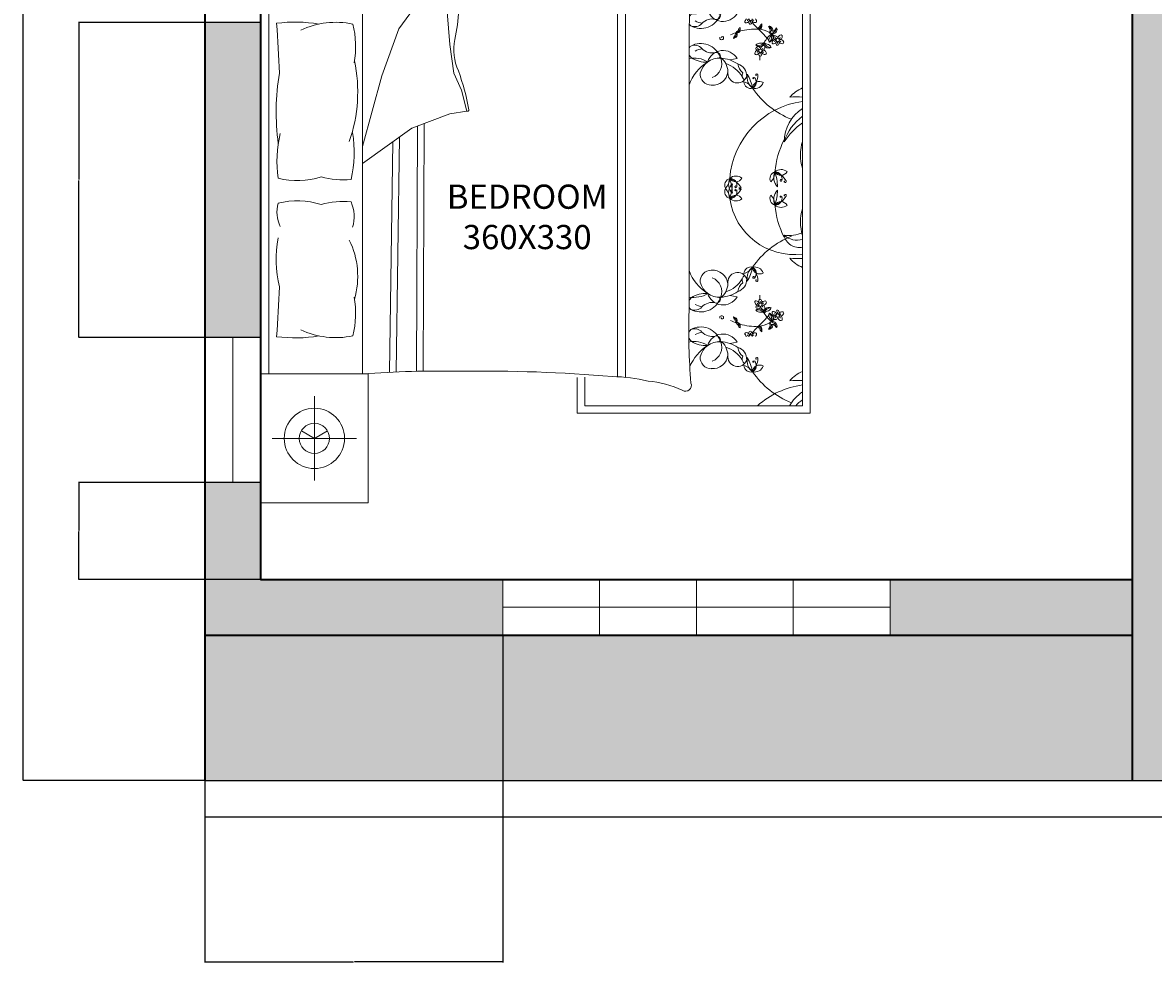
# Model space of a CAD drawing. Units: centimetres. Extents: x 2178 to 3635, y 1064 to 2635.
# Tile 1 of 9: x 2178 to 2645, y 1113 to 1502. Entities that reach past the tile are written whole.
import ezdxf

# ---------------------------------------------------------------- set-up
doc = ezdxf.new("R2010")
doc.units = ezdxf.units.CM
for name, color, linetype, lineweight in [('A-ANNO-DIMS', 2, 'Continuous', 18), ('A-AREA-IDEN', 7, 'Continuous', 18), ('A-FLOR', 7, 'Continuous', 25), ('A-FLOR-PATT', 95, 'Continuous', 13), ('A-FURN', 42, 'Continuous', 18), ('A-GLAZ', 4, 'Continuous', 18), ('A-WALL', 7, 'Continuous', 35)]:
    doc.layers.add(name, color=color, linetype=linetype, lineweight=lineweight)
doc.layers.add('A-WALL-PATT', color=18, linetype='Continuous', lineweight=13, true_color=0x000000)
doc.styles.get("Standard").update_dxf_attribs({"font": 'arial.ttf'})
doc.dimstyles.get("Standard").update_dxf_attribs({"dimtxt": 0.18, "dimasz": 0.18, "dimexe": 0.18, "dimexo": 0.0625, "dimgap": 0.09, "dimtad": 0, "dimtih": 1, "dimtoh": 1, "dimdec": 4, "dimzin": 0, "dimdsep": 46, "dimtxsty": 'Standard', "dimcen": 0.09, "dimadec": 0, "dimazin": 0, "dimtfac": 1, "dimtdec": 4, "dimtofl": 0, "dimtmove": 0, "dimatfit": 3, "dimfxl": 1, "dimtolj": 1, "dimtzin": 0, "dimarcsym": 0})

# ---------------------------------------------------------------- blocks, each defined once
blk = doc.blocks.new('bed')
for p, q in [((2798.77, 2937.13), (3098.77, 2937.13)), ((2858.77, 2937.13), (2858.77, 2854.79)), ((2828.77, 2892.53), (2828.77, 2931.73)), ((3038.77, 2933.28), (2858.77, 2933.28)), ((3068.77, 2892.53), (3068.77, 2931.73)), ((2848.37, 2912.13), (2809.17, 2912.13)), ((3049.17, 2912.13), (3088.37, 2912.13)), ((2858.77, 2889.72), (3038.77, 2889.72)), ((2900.44, 2880.8), (2933.16, 2889.72)), ((2941.19, 2889.72), (2924.75, 2866.84)), ((2878.57, 2872.91), (2900.44, 2880.8)), ((2867.02, 2864.41), (2878.57, 2872.91)), ((3037.85, 2874.18), (2928.92, 2872.64)), ((3037.97, 2877.26), (2931.16, 2875.76)), ((2924.75, 2866.84), (2918.06, 2849.23)), ((2856.09, 2851.66), (2867.02, 2864.41)), ((3037.71, 2861.65), (2922.6, 2861.18)), ((3037.69, 2864.73), (2923.78, 2864.28)), ((2858.52, 2849.23), (2856.09, 2851.66)), ((2870.67, 2850.44), (2858.52, 2849.23)), ((2885.86, 2849.23), (2870.67, 2850.44)), ((2899.23, 2847.41), (2885.86, 2849.23)), ((2907.13, 2843.76), (2899.23, 2847.41)), ((2918.06, 2849.23), (2916.85, 2841.33)), ((2916.85, 2841.33), (2907.13, 2843.76)), ((2838.37, 2790.07), (2855.34, 2790.07)), ((2838.37, 2682), (2838.37, 2790.07)), ((3040.44, 2790.07), (3057.08, 2790.07)), ((3057.08, 2790.07), (3057.08, 2682)), ((2855.33, 2786.59), (2841.85, 2786.59)), ((2841.85, 2786.59), (2841.85, 2685.48)), ((3053.6, 2786.59), (3040.38, 2786.59)), ((3053.6, 2685.48), (3053.6, 2786.59)), ((3040.42, 2767.62), (2855.31, 2767.62)), ((3040.13, 2771.36), (2855.32, 2771.36)), ((3009.67, 2738.15), (2887.87, 2738.15)), ((2871.41, 2715.89), (2870.75, 2719.28)), ((2892.38, 2715.89), (2893.04, 2719.28)), ((3003.07, 2715.89), (3002.41, 2719.28)), ((3024.04, 2715.89), (3024.7, 2719.28)), ((2841.85, 2685.48), (3053.6, 2685.48)), ((3057.08, 2682), (2838.37, 2682))]:
    blk.add_line(p, q)
for points in [[(2858.77, 2887.13), (2798.77, 2887.13), (2798.77, 2937.13)], [(3038.77, 2937.13), (3038.77, 2887.13), (3098.77, 2887.13), (3098.77, 2937.13)], [(2828.77, 2912.13), (2832.27, 2918.19)], [(3068.77, 2912.13), (3065.27, 2918.19)], [(2828.77, 2912.13), (2832.27, 2906.07)], [(3068.77, 2912.13), (3065.27, 2906.07)]]:
    blk.add_lwpolyline(points)
for points in [[(2876, 2929.65, 0.074897), (2876.37, 2910.06, -0.472817)], [(2947.37, 2908.96, 0.14099), (2947.97, 2928.95, 0.235245)], [(2960.18, 2908.96, -0.14099), (2959.58, 2928.95, -0.235245)], [(3021.54, 2929.65, -0.074897), (3021.18, 2910.06, 0.472817)], [(2855.46, 2824.19, 0.001242), (2855.31, 2767.26, -0.127202), (2849.3, 2738.9)], [(3040.05, 2773.72, 0.056112), (3042.23, 2757.21, 0.095341), (3046.45, 2741.32)]]:
    blk.add_lwpolyline(points, format="xyb")
for centre, radius in [((2828.77, 2912.13), 14), ((3068.77, 2912.13), 14), ((2828.77, 2912.13), 7), ((3068.77, 2912.13), 7), ((2888.74, 2705.02), 0.764), ((3006.71, 2705.02), 0.764), ((2883.74, 2696.97), 0.764), ((3011.71, 2696.97), 0.764)]:
    blk.add_circle(centre, radius)
for centre, radius, start, end in [((2917.11, 2821.09), 108.8, 82.2196, 99.497), ((2985.93, 2877.16), 52.74, 76.3427, 101.1841), ((3041.36, 5784.66), 2859.79, 266.68521, 267.14978), ((2940.09, 2876.08), 53.46, 81.5249, 103.96), ((2963.69, 2914.69), 14.84, 63.3437, 106.1026), ((2856.18, 5784.66), 2859.79, 272.85022, 273.31479), ((2914.22, 2902.19), 38.67, 155.1316, 191.7583), ((2983.32, 2902.19), 38.67, 348.2417, 24.8684), ((2912, 2898.93), 36.76, 354.0129, 15.8293), ((2995.54, 2898.93), 36.76, 164.1707, 185.9871), ((2886.7, 2933.16), 40.2, 255.1039, 281.0369), ((2907.87, 2961.74), 69.73, 258.0397, 289.2615), ((2936.1, 2946.52), 52.9, 259.8617, 283.6238), ((2965.7, 2909.52), 15.9, 245.0183, 288.5407), ((2993.49, 2930.2), 38.19, 243.8761, 286.1746), ((3010.84, 2933.16), 40.2, 258.9631, 284.8961), ((3576.57, 2853.06), 539.05, 176.1, 180.9282), ((2581.02, 2844.2), 275.17, 355.8294, 1.553), ((2861.22, 2957.89), 113.22, 267.4519, 281.3392), ((2888.28, 2822.94), 24.42, 66.2616, 101.3392), ((2937.68, 2954.7), 116.34, 250.1194, 259.3383), ((2916.17, 2841.09), 0.724, 268.8623, 19.7536), ((3740.68, 2833.46), 703.17, 179.11454, 184.87351), ((3044.17, 2739.79), 2.73, 246.5219, 33.8264), ((2852.06, 2739.09), 2.77, 183.98, 297.3412), ((2884.29, 2425.86), 312.3, 89.3433, 95.6887), ((2850.89, 2717.02), 22.71, 33.6671, 63.2997), ((2881.32, 2730.53), 11.57, 145.785, 184.7304), ((2859.22, 2735.93), 12.43, 328.8218, 9.1554), ((2874.61, 2734.83), 3.61, 120.0293, 142.325), ((2868.85, 2732.7), 9.56, 289.2822, 29.1751), ((2873.09, 2735.54), 4.49, 311.5653, 23.8354), ((2874.61, 2734.83), 3.61, 44.4517, 63.558), ((2894.94, 2732.7), 9.56, 150.8249, 250.7178), ((2890.7, 2735.54), 4.49, 156.1646, 228.4347), ((2889.17, 2734.83), 3.61, 113.229, 135.5483), ((2889.17, 2734.83), 3.61, 37.675, 66.7144), ((2882.46, 2730.53), 11.57, 355.2696, 34.215), ((2904.56, 2735.93), 12.43, 169.7133, 211.1782), ((2912.89, 2717.02), 22.71, 111.4941, 146.3329), ((2982.56, 2717.02), 22.71, 33.6671, 68.5059), ((3012.99, 2730.53), 11.57, 145.785, 184.7304), ((2990.89, 2735.93), 12.43, 328.8218, 10.2867), ((3006.28, 2734.83), 3.61, 113.2856, 142.325), ((3000.51, 2732.7), 9.56, 289.2822, 29.1751), ((3006.28, 2734.83), 3.61, 44.4517, 66.7144), ((3004.75, 2735.54), 4.49, 311.5653, 23.8354), ((3018.86, 2446.37), 291.92, 85.2402, 91.8035), ((3026.6, 2732.7), 9.56, 150.8249, 250.7178), ((3022.36, 2735.54), 4.49, 156.1646, 228.4347), ((3020.84, 2734.83), 3.61, 106.6343, 135.5483), ((3020.84, 2734.83), 3.61, 37.675, 72.5814), ((3014.13, 2730.53), 11.57, 355.2696, 34.215), ((3036.23, 2735.93), 12.43, 169.249, 211.1782), ((3044.56, 2717.02), 22.71, 113.6453, 146.3329), ((2864.12, 2727.92), 5.07, 84.4856, 181.0538), ((2862.56, 2724.18), 9.02, 355.2933, 76.921), ((2880.15, 2727.58), 6.15, 131.5653, 195.1471), ((2867.4, 2730.97), 8.62, 7.436, 29.9149), ((2883.64, 2727.58), 6.15, 344.8529, 48.4347), ((2896.38, 2730.97), 8.62, 150.0851, 172.564), ((2901.22, 2724.18), 9.02, 103.079, 184.7067), ((2899.66, 2727.92), 5.07, 358.9462, 95.5144), ((2995.79, 2727.92), 5.07, 84.4856, 181.0538), ((2994.23, 2724.18), 9.02, 355.2933, 76.921), ((3011.81, 2727.58), 6.15, 131.5653, 195.1471), ((2999.07, 2730.97), 8.62, 7.436, 29.9149), ((3015.3, 2727.58), 6.15, 344.8529, 48.4347), ((3028.05, 2730.97), 8.62, 150.0851, 172.564), ((3032.89, 2724.18), 9.02, 103.079, 184.7067), ((3031.33, 2727.92), 5.07, 358.9462, 95.5144), ((2866.2, 2727.2), 7.17, 174.9449, 262.8857), ((2869.01, 2729.92), 6.96, 201.5819, 291.4221), ((2867.69, 2722.36), 7.46, 299.9085, 73.1337), ((2872.41, 2725.49), 1.86, 257.3041, 15.1471), ((2896.09, 2722.36), 7.46, 106.8663, 240.0915), ((2891.37, 2725.49), 1.86, 164.8529, 282.6959), ((2894.77, 2729.92), 6.96, 248.5779, 338.4181), ((2897.59, 2727.2), 7.17, 277.1143, 5.0551), ((2997.86, 2727.2), 7.17, 174.9449, 262.8857), ((3000.68, 2729.92), 6.96, 201.5819, 291.4221), ((2999.36, 2722.36), 7.46, 299.9085, 73.1337), ((3004.08, 2725.49), 1.86, 257.3041, 15.1471), ((3027.76, 2722.36), 7.46, 106.8663, 240.0915), ((3023.04, 2725.49), 1.86, 164.8529, 282.6959), ((3026.44, 2729.92), 6.96, 248.5779, 338.4181), ((3029.25, 2727.2), 7.17, 277.1143, 5.0551), ((2864.55, 2715.65), 4.5, 80.264, 250.8688), ((2855.62, 2725.56), 14.16, 301.2614, 341.7045), ((2864.95, 2728.79), 8.71, 272.3591, 324.0401), ((2855.49, 2724.42), 16.1, 326.2883, 356.5076), ((2881.32, 2730.53), 11.57, 212.7011, 216.3445), ((2882.75, 2722.67), 0.578, 102.7051, 280.4384), ((2882.69, 2723.02), 0.94, 280.4384, 100.4136), ((2882.46, 2730.53), 11.57, 323.6555, 327.2989), ((2898.83, 2728.79), 8.71, 215.9599, 267.6409), ((2908.3, 2724.42), 16.1, 183.4924, 213.7117), ((2908.16, 2725.56), 14.16, 198.2955, 238.7386), ((2899.24, 2715.65), 4.5, 289.1312, 99.736), ((2951.17, 2718.35), 3.25, 63.0274, 163.8037), ((2947.89, 2725.94), 6.69, 271.4585, 315.3727), ((2954.28, 2718.35), 3.25, 16.1963, 116.9726), ((2957.56, 2725.94), 6.69, 224.6273, 268.5415), ((2996.21, 2715.65), 4.5, 80.264, 250.8688), ((2987.29, 2725.56), 14.16, 301.2614, 341.7045), ((2996.62, 2728.79), 8.71, 272.3591, 324.0401), ((2987.15, 2724.42), 16.1, 326.2883, 356.5076), ((3012.99, 2730.53), 11.57, 212.7011, 216.3445), ((3012.76, 2723.02), 0.94, 79.5864, 259.5616), ((3012.7, 2722.67), 0.578, 259.5616, 77.2949), ((3014.13, 2730.53), 11.57, 323.6555, 327.2989), ((3030.5, 2728.79), 8.71, 215.9599, 267.6409), ((3039.96, 2724.42), 16.1, 183.4924, 213.7117), ((3039.83, 2725.56), 14.16, 198.2955, 238.7386), ((3030.9, 2715.65), 4.5, 289.1312, 99.736), ((2863.47, 2717), 5.62, 265.969, 344.3045), ((2869.52, 2709.53), 5.99, 96.1662, 141.5825), ((2879.44, 2713.73), 1.58, 101.3256, 154.4621), ((2877.17, 2719.07), 4.74, 280.2588, 300.656), ((2903.55, 2707.57), 24.85, 163.5842, 183.8277), ((2876.15, 2719.06), 4.82, 308.2101, 316.3071), ((2879.11, 2715.89), 1.44, 278.3432, 4.2869), ((2878.31, 2717.16), 2.51, 300.656, 332.6341), ((2880.2, 2715.5), 0.611, 55.7657, 157.4417), ((2903.55, 2707.57), 24.85, 153.0032, 159.8941), ((2881.15, 2716.07), 0.611, 84.3784, 186.0543), ((2880.58, 2718.52), 2.51, 269.1859, 301.164), ((2881.32, 2717.22), 1.44, 237.5332, 323.4768), ((2879.92, 2721.32), 4.82, 285.5129, 293.6099), ((2883.07, 2715.9), 1.58, 87.3579, 140.4944), ((2879.43, 2720.42), 4.74, 301.164, 321.5612), ((2875.57, 2721.25), 8.46, 324.6898, 333.4936), ((2894.26, 2709.53), 5.99, 38.4175, 83.8338), ((2900.32, 2717), 5.62, 195.6955, 274.031), ((2951.1, 2680.2), 39.18, 94.4623, 172.255), ((2951.27, 2716.33), 4.34, 137.7873, 219.1145), ((2946.34, 2716.47), 3.27, 298.5391, 58.3627), ((2951.26, 2719.13), 3.2, 177.7585, 283.852), ((2950.61, 2713.61), 6.19, 45.5411, 114.3101), ((2956.25, 2745.4), 27.41, 252.593, 267.2582), ((2957.43, 2722.47), 9.91, 198.9159, 238.011), ((2954.84, 2713.61), 6.19, 65.6899, 134.4589), ((2949.2, 2745.4), 27.41, 272.7418, 287.407), ((2951.92, 2716.43), 0.424, 283.852, 219.9245), ((2952.44, 2714.47), 0.487, 238.011, 71.5592), ((2952.52, 2714.71), 0.236, 71.5592, 188.0167), ((2953.01, 2714.47), 0.487, 108.4408, 301.989), ((2952.93, 2714.71), 0.236, 351.9833, 108.4408), ((2953.49, 2716.59), 0.255, 320.1909, 256.0209), ((2948.02, 2722.47), 9.91, 301.989, 341.0841), ((2954.19, 2719.13), 3.2, 256.148, 2.2415), ((2959.11, 2716.47), 3.27, 121.6373, 241.4609), ((2954.18, 2716.33), 4.34, 320.8855, 42.2127), ((2953.08, 2689.24), 30.32, 352.8636, 81.8197), ((2995.13, 2717), 5.62, 265.969, 344.3045), ((3001.19, 2709.53), 5.99, 96.1662, 141.5825), ((3012.38, 2715.9), 1.58, 39.5056, 92.6421), ((3016.02, 2720.42), 4.74, 218.4388, 238.836), ((3019.88, 2721.25), 8.46, 206.5064, 215.3102), ((3014.13, 2717.22), 1.44, 216.5232, 302.4668), ((3014.87, 2718.52), 2.51, 238.836, 270.8141), ((3015.53, 2721.32), 4.82, 246.3901, 254.4871), ((2991.9, 2707.57), 24.85, 20.1059, 26.9968), ((3014.3, 2716.07), 0.611, 353.9457, 95.6216), ((3016.34, 2715.89), 1.44, 175.7131, 261.6568), ((3015.25, 2715.5), 0.611, 22.5583, 124.2343), ((3017.14, 2717.16), 2.51, 207.3659, 239.344), ((2991.9, 2707.57), 24.85, 356.1723, 16.4158), ((3019.3, 2719.06), 4.82, 223.6929, 231.7899), ((3018.28, 2719.07), 4.74, 239.344, 259.7412), ((3016.01, 2713.73), 1.58, 25.5379, 78.6744), ((3031.98, 2717), 5.62, 195.6955, 274.031), ((3025.93, 2709.53), 5.99, 38.4175, 83.8338), ((2860.73, 2709.42), 3.25, 92.9516, 193.728), ((2854.09, 2714.37), 6.69, 301.3827, 345.2969), ((2862.6, 2705.03), 6.19, 75.4653, 144.2343), ((2851.64, 2735.41), 27.41, 282.5173, 297.1824), ((2863.62, 2710.77), 2.76, 63.9755, 143.2681), ((2874.99, 2710.74), 1.27, 101.5637, 142.6358), ((2873.93, 2709.56), 0.764, 273.2768, 86.7232), ((2874.82, 2710.28), 0.73, 91.1081, 181.8675), ((2875.59, 2708.82), 1.58, 80.3487, 133.6538), ((2873.96, 2711.74), 1.84, 288.7263, 352.5032), ((2875.3, 2707.17), 2.5, 83.0852, 105.7171), ((2875.21, 2711.65), 0.59, 345.2356, 144.9248), ((2875.75, 2709.72), 0.658, 317.6792, 80.3487), ((2878.27, 2722.86), 8.46, 268.3264, 277.1302), ((2900.16, 2710.77), 2.76, 36.7319, 116.0245), ((2901.18, 2705.03), 6.19, 35.7657, 104.5347), ((2912.15, 2735.41), 27.41, 242.8176, 257.4827), ((2903.05, 2709.42), 3.25, 346.272, 87.0484), ((2909.69, 2714.37), 6.69, 194.7031, 238.6173), ((2992.4, 2709.42), 3.25, 92.9516, 193.728), ((2985.76, 2714.37), 6.69, 301.3827, 345.2969), ((2994.27, 2705.03), 6.19, 75.4653, 144.2343), ((2983.3, 2735.41), 27.41, 282.5173, 297.1824), ((2995.29, 2710.77), 2.76, 63.9755, 143.2681), ((3017.18, 2722.86), 8.46, 262.8698, 271.6736), ((3019.7, 2709.72), 0.658, 99.6513, 222.3208), ((3019.86, 2708.82), 1.58, 46.3462, 99.6513), ((3020.24, 2711.65), 0.59, 35.0752, 194.7644), ((3021.49, 2711.74), 1.84, 187.4968, 251.2737), ((3020.15, 2707.17), 2.5, 74.2829, 96.9148), ((3020.63, 2710.28), 0.73, 358.1325, 88.8919), ((3020.46, 2710.74), 1.27, 37.3642, 78.4363), ((3021.52, 2709.56), 0.764, 93.2768, 266.7232), ((3031.83, 2710.77), 2.76, 36.7319, 116.0245), ((3032.85, 2705.03), 6.19, 35.7657, 104.5347), ((3043.81, 2735.41), 27.41, 242.8176, 257.4827), ((3041.36, 2714.37), 6.69, 194.7031, 238.6173), ((3034.72, 2709.42), 3.25, 346.272, 87.0484), ((2812.68, 2680.2), 39.18, 7.745, 41.8856), ((2879.7, 2676.32), 39.18, 124.3865, 158.5908), ((2861.82, 2707.73), 4.34, 167.7115, 249.0387), ((2857.48, 2705.38), 3.27, 328.4633, 88.2869), ((2864.1, 2716.11), 9.91, 228.8402, 267.9352), ((2860.42, 2710.14), 3.2, 207.6827, 313.7762), ((2862.34, 2708.13), 0.424, 313.7762, 249.7183), ((2863.71, 2706.94), 0.236, 101.4834, 217.9409), ((2863.76, 2706.7), 0.487, 267.9352, 101.4834), ((2874.97, 2708.15), 1.26, 217.7621, 259.0403), ((2876.33, 2709.83), 2.32, 203.4276, 227.6104), ((2875.31, 2710.12), 1.25, 229.7889, 317.6792), ((2873.9, 2707.47), 1.78, 355.053, 68.3618), ((2875.09, 2707.37), 0.586, 232.4737, 355.053), ((2857.98, 2686.43), 28.48, 43.1541, 52.0459), ((2877.65, 2703.63), 1.58, 101.3256, 154.4621), ((2875.39, 2708.98), 4.74, 280.2588, 300.656), ((2876.48, 2712.77), 8.46, 268.3264, 277.1302), ((2874.36, 2708.97), 4.82, 308.2101, 316.3071), ((2877.32, 2705.8), 1.44, 278.3432, 4.2869), ((2876.52, 2707.06), 2.51, 300.656, 332.6341), ((2878.41, 2705.4), 0.611, 55.7657, 157.4417), ((2891.17, 2706.94), 12.46, 184.756, 209.2041), ((2909.1, 2733.46), 40.99, 222.2412, 232.1744), ((2884.75, 2705.38), 2.12, 272.8499, 356.1226), ((2882.89, 2706.16), 3.48, 304.5369, 16.3699), ((2883.26, 2704.56), 2.05, 321.7607, 7.9252), ((2887.73, 2705.18), 2.46, 127.3105, 187.9252), ((2884.34, 2705.45), 2.53, 355.0106, 41.658), ((2892.45, 2690.4), 14.94, 113.0501, 113.8477), ((2888.54, 2702.71), 2.41, 104.7558, 148.0499), ((2887.18, 2704.44), 1.51, 247.4086, 351.4386), ((2887.9, 2706.08), 1.04, 126.1046, 271.4281), ((2887.78, 2706.37), 0.749, 353.7526, 131.7054), ((2887.61, 2704.38), 0.506, 262.906, 7.132), ((2887.08, 2705.48), 1.05, 0.0645, 61.1507), ((2887.33, 2706.37), 1.2, 311.8413, 355.7877), ((2889.78, 2703.61), 1.26, 151.2196, 259.0403), ((2889.8, 2706.2), 1.27, 101.5637, 176.365), ((2889.63, 2705.74), 0.73, 91.1081, 181.8675), ((2891.14, 2705.29), 2.32, 203.4276, 227.6104), ((2890.41, 2704.28), 1.58, 80.3487, 133.6538), ((2890.12, 2705.58), 1.25, 229.7889, 317.6792), ((2888.77, 2707.2), 1.84, 288.7263, 352.5032), ((2888.71, 2702.93), 1.78, 355.053, 68.3618), ((2890.11, 2702.63), 2.5, 83.0852, 105.7171), ((2890.02, 2707.11), 0.59, 345.2356, 144.9248), ((2890.56, 2705.18), 0.658, 317.6792, 80.3487), ((2892.45, 2690.4), 14.94, 87.1071, 94.7585), ((2900.02, 2706.7), 0.487, 78.5166, 272.0648), ((2899.68, 2716.11), 9.91, 272.0648, 311.1598), ((2900.07, 2706.94), 0.236, 322.0591, 78.5166), ((2903.37, 2710.14), 3.2, 226.2238, 332.3173), ((2901.49, 2708.3), 0.255, 290.2667, 226.2271), ((2906.3, 2705.38), 3.27, 91.7131, 211.5367), ((2901.96, 2707.73), 4.34, 290.9613, 12.2885), ((2884.08, 2676.32), 39.18, 21.4092, 55.6135), ((3011.37, 2676.32), 39.18, 124.3865, 158.5908), ((2993.49, 2707.73), 4.34, 167.7115, 249.0387), ((2992.08, 2710.14), 3.2, 207.6827, 313.7762), ((2995.76, 2716.11), 9.91, 228.8402, 267.9352), ((2989.15, 2705.38), 3.27, 328.4633, 88.2869), ((2994.01, 2708.13), 0.424, 313.7762, 249.7183), ((2995.38, 2706.94), 0.236, 101.4834, 217.9409), ((2995.43, 2706.7), 0.487, 267.9352, 101.4834), ((3003, 2690.4), 14.94, 85.2415, 92.8929), ((3004.89, 2705.18), 0.658, 99.6513, 222.3208), ((3005.33, 2705.58), 1.25, 222.3208, 310.2111), ((3005.04, 2704.28), 1.58, 46.3462, 99.6513), ((3005.43, 2707.11), 0.59, 35.0752, 194.7644), ((3006.68, 2707.2), 1.84, 187.4968, 251.2737), ((3006.74, 2702.93), 1.78, 111.6382, 184.947), ((3005.34, 2702.63), 2.5, 74.2829, 96.9148), ((3005.82, 2705.74), 0.73, 358.1325, 88.8919), ((3004.31, 2705.29), 2.32, 312.3896, 336.5724), ((3005.65, 2706.2), 1.27, 3.635, 78.4363), ((3005.67, 2703.61), 1.26, 280.9597, 28.7804), ((3008.27, 2704.44), 1.51, 188.5614, 292.5914), ((3007.67, 2706.37), 0.749, 48.2946, 186.2474), ((3008.12, 2706.37), 1.2, 184.2123, 228.1587), ((3008.37, 2705.48), 1.05, 118.8493, 179.9355), ((3007.84, 2704.38), 0.506, 172.868, 277.094), ((3007.55, 2706.08), 1.04, 268.5719, 53.8954), ((3006.91, 2702.71), 2.41, 31.9501, 75.2442), ((3011.11, 2705.45), 2.53, 138.342, 184.9894), ((3010.7, 2705.38), 2.12, 183.8774, 267.1501), ((3003, 2690.4), 14.94, 66.1523, 66.9499), ((3012.56, 2706.16), 3.48, 163.6301, 235.4631), ((3007.72, 2705.18), 2.46, 352.0748, 52.6895), ((3012.19, 2704.56), 2.05, 172.0748, 218.2393), ((2986.35, 2733.46), 40.99, 307.8256, 317.7588), ((3004.28, 2706.94), 12.46, 330.7959, 355.244), ((3037.47, 2686.43), 28.48, 127.9541, 136.8459), ((3017.04, 2705.4), 0.611, 22.5583, 124.2343), ((3018.13, 2705.8), 1.44, 175.7131, 261.6568), ((3018.93, 2707.06), 2.51, 207.3659, 239.344), ((3021.09, 2708.97), 4.82, 223.6929, 231.7899), ((3020.06, 2708.98), 4.74, 239.344, 259.7412), ((3018.97, 2712.77), 8.46, 262.8698, 271.6736), ((3017.8, 2703.63), 1.58, 25.5379, 78.6744), ((3020.14, 2710.12), 1.25, 222.3208, 310.2111), ((3021.55, 2707.47), 1.78, 111.6382, 184.947), ((3020.36, 2707.37), 0.586, 184.947, 307.5263), ((3019.12, 2709.83), 2.32, 312.3896, 336.5724), ((3020.48, 2708.15), 1.26, 280.9597, 322.2379), ((3031.69, 2706.7), 0.487, 78.5166, 272.0648), ((3031.35, 2716.11), 9.91, 272.0648, 311.1598), ((3031.74, 2706.94), 0.236, 322.0591, 78.5166), ((3035.03, 2710.14), 3.2, 226.2238, 332.3173), ((3033.16, 2708.3), 0.255, 290.2667, 226.2271), ((3037.97, 2705.38), 3.27, 91.7131, 211.5367), ((3033.63, 2707.73), 4.34, 290.9613, 12.2885), ((3015.75, 2676.32), 39.18, 21.4092, 55.6135), ((3082.77, 2680.2), 39.18, 138.1144, 172.255), ((2878.18, 2700.87), 0.853, 146.8636, 236.9021), ((2890.21, 2719.66), 22.32, 235.1882, 238.8844), ((2879.65, 2702.11), 2.31, 199.4799, 267.6828), ((2879.39, 2701.23), 1.99, 212.8155, 277.3992), ((2878.23, 2699.91), 2.31, 266.9701, 338.2913), ((2879.13, 2701.31), 0.883, 238.8844, 314.2646), ((2878.94, 2699.33), 1.99, 280.3057, 17.1958), ((2878.77, 2699.13), 0.883, 306.3746, 21.7548), ((2880.21, 2699.7), 0.666, 19.3605, 201.7548), ((2880.22, 2700.2), 0.666, 311.8703, 134.2646), ((2892.74, 2694.13), 13.31, 153.7819, 158.2913), ((2882.15, 2703.22), 3.48, 247.2305, 319.0635), ((2881, 2702.05), 2.05, 264.4544, 310.6188), ((2891.17, 2706.94), 12.46, 214.0033, 222.4917), ((2882.5, 2701.23), 2.12, 218.3208, 298.8162), ((2892.45, 2690.4), 14.94, 120.544, 139.818), ((2882.9, 2698.03), 1.04, 126.1046, 271.4281), ((2882.78, 2698.31), 0.749, 353.7526, 131.7054), ((2883.94, 2698.62), 2.46, 70.0041, 130.6188), ((2882.35, 2701.62), 2.53, 297.7043, 344.3516), ((2884.8, 2698.15), 1.27, 101.5637, 176.365), ((2883.78, 2699.15), 1.84, 288.7263, 352.5032), ((2885.03, 2699.06), 0.59, 345.2356, 144.9248), ((2883.69, 2701.61), 2.05, 8.7227, 54.8872), ((2883.8, 2699.97), 3.48, 0.278, 72.111), ((2885.36, 2701.25), 2.12, 20.5253, 88.5375), ((2888.15, 2702.29), 2.46, 188.7227, 249.3375), ((2887.13, 2703.59), 0.757, 148.0499, 225.6268), ((2884.99, 2701.06), 2.53, 334.9899, 21.6373), ((2889.9, 2702.83), 0.586, 232.4737, 355.053), ((2948.18, 2697.36), 3.25, 63.0274, 163.8037), ((2944.89, 2704.96), 6.69, 271.4585, 315.3727), ((2947.61, 2692.63), 6.19, 45.5411, 114.3101), ((2957.84, 2692.63), 6.19, 65.6899, 134.4589), ((2957.27, 2697.36), 3.25, 16.1963, 116.9726), ((2960.56, 2704.96), 6.69, 224.6273, 268.5415), ((3005.55, 2702.83), 0.586, 184.947, 307.5263), ((3010.46, 2701.06), 2.53, 158.3627, 205.0101), ((3010.09, 2701.25), 2.12, 91.4625, 159.4747), ((3011.65, 2699.97), 3.48, 107.889, 179.722), ((3007.3, 2702.29), 2.46, 290.6625, 351.2773), ((3008.32, 2703.59), 0.757, 314.3732, 31.9501), ((3011.76, 2701.61), 2.05, 125.1128, 171.2773), ((3010.42, 2699.06), 0.59, 35.0752, 194.7644), ((3011.67, 2699.15), 1.84, 187.4968, 251.2737), ((3003, 2690.4), 14.94, 40.182, 59.456), ((3011.51, 2698.62), 2.46, 49.3812, 109.9959), ((3013.3, 2703.22), 3.48, 220.9365, 292.7695), ((3013.1, 2701.62), 2.53, 195.6484, 242.2957), ((3010.65, 2698.15), 1.27, 3.635, 78.4363), ((3012.67, 2698.31), 0.749, 48.2946, 186.2474), ((3012.95, 2701.23), 2.12, 241.1838, 321.6792), ((3012.55, 2698.03), 1.04, 268.5719, 53.8954), ((3014.45, 2702.05), 2.05, 229.3812, 275.5456), ((3004.28, 2706.94), 12.46, 317.5083, 325.9967), ((3016.51, 2699.33), 1.99, 162.8042, 259.6943), ((3015.23, 2700.2), 0.666, 45.7354, 228.1297), ((3015.24, 2699.7), 0.666, 338.2452, 160.6395), ((3002.71, 2694.13), 13.31, 21.7087, 26.2181), ((3017.22, 2699.91), 2.31, 201.7087, 273.0299), ((3016.32, 2701.31), 0.883, 225.7354, 301.1156), ((3016.68, 2699.13), 0.883, 158.2452, 233.6254), ((3016.06, 2701.23), 1.99, 262.6008, 327.1845), ((3015.8, 2702.11), 2.31, 272.3172, 340.5201), ((3005.24, 2719.66), 22.32, 301.1156, 304.8118), ((3017.27, 2700.87), 0.853, 303.0979, 33.1364), ((2866.06, 2716.39), 22.32, 302.6784, 306.3746), ((2878.82, 2698.08), 0.853, 214.3538, 304.3923), ((2882.14, 2695.53), 0.757, 148.0499, 225.6268), ((2883.54, 2694.66), 2.41, 104.7558, 148.0499), ((2882.19, 2696.38), 1.51, 247.4086, 351.4386), ((2882.61, 2696.32), 0.506, 262.906, 7.132), ((2882.08, 2697.42), 1.05, 0.0645, 61.1507), ((2882.33, 2698.32), 1.2, 311.8413, 355.7877), ((2884.78, 2695.55), 1.26, 151.2196, 259.0403), ((2884.63, 2697.69), 0.73, 91.1081, 181.8675), ((2886.15, 2697.23), 2.32, 203.4276, 227.6104), ((2885.41, 2696.22), 1.58, 80.3487, 133.6538), ((2885.13, 2697.53), 1.25, 229.7889, 317.6792), ((2883.72, 2694.88), 1.78, 355.053, 68.3618), ((2885.11, 2694.58), 2.5, 83.0852, 105.7171), ((2884.9, 2694.78), 0.586, 232.4737, 355.053), ((2885.56, 2697.13), 0.658, 317.6792, 80.3487), ((2931.45, 2674.95), 19.09, 91.272, 146.5383), ((2938.32, 2671.39), 23.79, 107.8504, 143.6964), ((2950.82, 2664.7), 35.39, 124.0123, 144.053), ((2948.1, 2659.21), 39.18, 94.4623, 117.4146), ((2948.27, 2695.35), 4.34, 137.7873, 219.1145), ((2943.34, 2695.48), 3.27, 298.5391, 58.3627), ((2948.26, 2698.14), 3.2, 177.7585, 283.852), ((2954.43, 2701.48), 9.91, 198.9159, 238.011), ((2953.26, 2724.42), 27.41, 252.593, 267.2582), ((2948.92, 2695.44), 0.424, 283.852, 219.9245), ((2949.44, 2693.49), 0.487, 238.011, 71.5592), ((2949.52, 2693.73), 0.236, 71.5592, 188.0167), ((2952.19, 2724.42), 27.41, 272.7418, 287.407), ((2956.01, 2693.49), 0.487, 108.4408, 301.989), ((2955.93, 2693.73), 0.236, 351.9833, 108.4408), ((2956.49, 2695.61), 0.255, 320.1909, 256.0209), ((2951.02, 2701.48), 9.91, 301.989, 341.0841), ((2957.19, 2698.14), 3.2, 256.148, 2.2415), ((2962.11, 2695.48), 3.27, 121.6373, 241.4609), ((2957.18, 2695.35), 4.34, 320.8855, 42.2127), ((2957.35, 2659.21), 39.18, 62.5854, 85.5377), ((2957, 2692.01), 17.54, 338.117, 6.6195), ((2973.09, 2687.13), 7.03, 346.3898, 79.0739), ((2967.81, 2688.1), 8.89, 342.8609, 41.9049), ((3009.89, 2697.13), 0.658, 99.6513, 222.3208), ((3010.32, 2697.53), 1.25, 222.3208, 310.2111), ((3010.04, 2696.22), 1.58, 46.3462, 99.6513), ((3011.73, 2694.88), 1.78, 111.6382, 184.947), ((3010.55, 2694.78), 0.586, 184.947, 307.5263), ((3010.34, 2694.58), 2.5, 74.2829, 96.9148), ((3010.82, 2697.69), 0.73, 358.1325, 88.8919), ((3009.3, 2697.23), 2.32, 312.3896, 336.5724), ((3010.67, 2695.55), 1.26, 280.9597, 28.7804), ((3013.26, 2696.38), 1.51, 188.5614, 292.5914), ((3013.12, 2698.32), 1.2, 184.2123, 228.1587), ((3013.37, 2697.42), 1.05, 118.8493, 179.9355), ((3012.84, 2696.32), 0.506, 172.868, 277.094), ((3011.91, 2694.66), 2.41, 31.9501, 75.2442), ((3013.31, 2695.53), 0.757, 314.3732, 31.9501), ((3029.39, 2716.39), 22.32, 233.6254, 237.3216), ((3016.63, 2698.08), 0.853, 235.6077, 325.6462), ((2832.33, 2674.95), 19.09, 33.4617, 60.1116), ((2825.46, 2671.39), 23.79, 36.3036, 46.4814), ((2843.02, 2679.37), 15.93, 22.5547, 48.9546), ((2799.39, 2687.93), 54.2, 357.4081, 3.6519), ((2920.76, 2679.37), 15.93, 131.0454, 157.4453), ((2964.39, 2687.93), 54.2, 176.3481, 182.5919), ((2931.06, 2687.93), 54.2, 357.4081, 3.6519), ((2974.69, 2679.37), 15.93, 22.5547, 48.9546), ((3052.43, 2679.37), 15.93, 131.0454, 157.4453), ((3096.06, 2687.93), 54.2, 176.3481, 182.5919), ((3063.12, 2674.95), 19.09, 119.8884, 146.5383), ((3069.99, 2671.39), 23.79, 133.5186, 143.6964), ((2937.15, 2664.88), 21.54, 73.5431, 107.0202), ((2945.68, 2653.78), 31.85, 94.3787, 95.6357), ((2962.46, 2631.95), 56.92, 109.7217, 109.9028), ((2968.3, 2664.88), 21.54, 72.9798, 106.4569), ((2959.77, 2653.78), 31.85, 84.3643, 85.6213), ((2942.99, 2631.95), 56.92, 70.0972, 70.2783)]:
    blk.add_arc(centre, radius, start, end)
blk = doc.blocks.new('WIN-1600-4LT')
for p, q in [((0, 23), (0, 0)), ((40, 23), (40, 0)), ((80, 23), (80, 0)), ((120, 23), (120, 0)), ((160, 23), (160, 0)), ((0, 11.5), (160, 11.5))]:
    blk.add_line(p, q)
blk = doc.blocks.new('WIN-0600')
for p, q in [((0, 60), (23, 60)), ((11.5, 60), (11.5, 0)), ((0, 0), (23, 0))]:
    blk.add_line(p, q)
blk = doc.blocks.new('*D46')
at = {"layer": 'A-ANNO-DIMS', "color": 0, "lineweight": -2, "transparency": 16777216}
for p, q in [((2253.6, 1248.53), (2253.6, 1173.41)), ((3559.6, 1248.53), (3559.6, 1173.41)), ((2253.78, 1173.59), (2906.25, 1173.59)), ((3559.42, 1173.59), (2906.95, 1173.59))]:
    blk.add_line(p, q, dxfattribs=at)
at = {"layer": 'A-ANNO-DIMS', "color": 0, "transparency": 16777216}
for points in [[(2253.78, 1173.62), (2253.78, 1173.56), (2253.6, 1173.59)], [(3559.42, 1173.62), (3559.42, 1173.56), (3559.6, 1173.59)]]:
    blk.add_solid(points, dxfattribs=at)
at = {"layer": 'Defpoints', "color": 0, "transparency": 16777216}
for p in [(2253.6, 1248.59), (3559.6, 1248.59), (2253.6, 1173.59)]:
    blk.add_point(p, dxfattribs=at)
at = {"layer": 'A-ANNO-DIMS', "color": 0, "transparency": 16777216, "insert": (2906.6, 1173.59), "char_height": 0.18, "attachment_point": 5}
blk.add_mtext('\\A1;1306', dxfattribs=at)
blk = doc.blocks.new('*D47')
at = {"layer": 'A-ANNO-DIMS', "color": 0, "lineweight": -2, "transparency": 16777216}
for p, q in [((2511.88, 2559.59), (2178.42, 2559.59)), ((2178.6, 2559.41), (2178.6, 1874.27)), ((2178.6, 1188.77), (2178.6, 1873.91)), ((2253.54, 1188.59), (2178.42, 1188.59))]:
    blk.add_line(p, q, dxfattribs=at)
at = {"layer": 'A-ANNO-DIMS', "color": 0, "transparency": 16777216}
for points in [[(2178.57, 2559.41), (2178.63, 2559.41), (2178.6, 2559.59)], [(2178.57, 1188.77), (2178.63, 1188.77), (2178.6, 1188.59)]]:
    blk.add_solid(points, dxfattribs=at)
at = {"layer": 'Defpoints', "color": 0, "transparency": 16777216}
for p in [(2178.6, 2559.59), (2511.95, 2559.59), (2253.6, 1188.59)]:
    blk.add_point(p, dxfattribs=at)
at = {"layer": 'A-ANNO-DIMS', "color": 0, "transparency": 16777216, "insert": (2178.6, 1874.09), "char_height": 0.18, "attachment_point": 5}
blk.add_mtext('\\A1;1371', dxfattribs=at)
blk = doc.blocks.new('*D69')
at = {"layer": 'A-ANNO-DIMS', "color": 0, "lineweight": -2, "transparency": 16777216}
for p, q in [((2276.54, 1311.59), (2201.42, 1311.59)), ((2201.6, 1311.41), (2201.6, 1291.77)), ((2201.6, 1271.77), (2201.6, 1291.41)), ((2276.54, 1271.59), (2201.42, 1271.59))]:
    blk.add_line(p, q, dxfattribs=at)
at = {"layer": 'A-ANNO-DIMS', "color": 0, "transparency": 16777216}
for points in [[(2201.57, 1311.41), (2201.63, 1311.41), (2201.6, 1311.59)], [(2201.57, 1271.77), (2201.63, 1271.77), (2201.6, 1271.59)]]:
    blk.add_solid(points, dxfattribs=at)
at = {"layer": 'Defpoints', "color": 0, "transparency": 16777216}
for p in [(2201.6, 1311.59), (2276.6, 1311.59), (2276.6, 1271.59)]:
    blk.add_point(p, dxfattribs=at)
at = {"layer": 'A-ANNO-DIMS', "color": 0, "transparency": 16777216, "insert": (2201.6, 1291.59), "char_height": 0.18, "attachment_point": 5}
blk.add_mtext('\\A1;40', dxfattribs=at)
blk = doc.blocks.new('*D70')
at = {"layer": 'A-ANNO-DIMS', "color": 0, "lineweight": -2, "transparency": 16777216}
for p, q in [((2276.54, 1501.59), (2201.42, 1501.59)), ((2201.6, 1501.41), (2201.6, 1436.77)), ((2201.6, 1371.77), (2201.6, 1436.41)), ((2276.54, 1371.59), (2201.42, 1371.59))]:
    blk.add_line(p, q, dxfattribs=at)
at = {"layer": 'A-ANNO-DIMS', "color": 0, "transparency": 16777216}
for points in [[(2201.57, 1501.41), (2201.63, 1501.41), (2201.6, 1501.59)], [(2201.57, 1371.77), (2201.63, 1371.77), (2201.6, 1371.59)]]:
    blk.add_solid(points, dxfattribs=at)
at = {"layer": 'Defpoints', "color": 0, "transparency": 16777216}
for p in [(2201.6, 1501.59), (2276.6, 1501.59), (2276.6, 1371.59)]:
    blk.add_point(p, dxfattribs=at)
at = {"layer": 'A-ANNO-DIMS', "color": 0, "transparency": 16777216, "insert": (2201.6, 1436.59), "char_height": 0.18, "attachment_point": 5}
blk.add_mtext('\\A1;130', dxfattribs=at)
blk = doc.blocks.new('*D75')
at = {"layer": 'A-ANNO-DIMS', "color": 0, "lineweight": -2, "transparency": 16777216}
for p, q in [((2253.6, 1248.53), (2253.6, 1113.41)), ((2376.6, 1248.53), (2376.6, 1113.41)), ((2253.78, 1113.59), (2314.82, 1113.59)), ((2376.42, 1113.59), (2315.39, 1113.59))]:
    blk.add_line(p, q, dxfattribs=at)
at = {"layer": 'A-ANNO-DIMS', "color": 0, "transparency": 16777216}
for points in [[(2253.78, 1113.62), (2253.78, 1113.56), (2253.6, 1113.59)], [(2376.42, 1113.62), (2376.42, 1113.56), (2376.6, 1113.59)]]:
    blk.add_solid(points, dxfattribs=at)
at = {"layer": 'Defpoints', "color": 0, "transparency": 16777216}
for p in [(2253.6, 1248.59), (2376.6, 1248.59), (2376.6, 1113.59)]:
    blk.add_point(p, dxfattribs=at)
at = {"layer": 'A-ANNO-DIMS', "color": 0, "transparency": 16777216, "insert": (2315.1, 1113.59), "char_height": 0.18, "attachment_point": 5}
blk.add_mtext('\\A1;123', dxfattribs=at)

msp = doc.modelspace()

# ---------------------------------------------------------------- hatches: boundary and pattern name
at = {"layer": 'A-FLOR-PATT'}
h = msp.add_hatch(color=256, dxfattribs=at)
h.dxf.hatch_style = 1
h.paths.add_polyline_path([(3559.605, 1741.59), (3395.605, 1741.59), (3395.605, 1623.59), (3559.605, 1623.59)])
h.paths.add_polyline_path([(3536.605, 1248.59), (3395.605, 1248.59), (3395.605, 1188.59), (3536.605, 1188.59)])
h.paths.add_polyline_path([(2636.605, 1248.59), (2253.605, 1248.59), (2253.605, 1188.59), (2636.605, 1188.59)])
at = {"layer": 'A-WALL-PATT'}
h = msp.add_hatch(color=256, dxfattribs=at)
h.dxf.hatch_style = 1
h.paths.add_polyline_path([(2276.605, 2499.59), (2253.605, 2499.59), (2253.605, 2476.59), (2276.605, 2476.59)])
h.paths.add_polyline_path([(2411.605, 2350.59), (2253.605, 2350.59), (2253.605, 2327.59), (2411.605, 2327.59)])
h.paths.add_polyline_path([(2276.605, 2252.59), (2253.605, 2252.59), (2253.605, 2020.59), (2276.605, 2020.59), (2276.605, 2093.59), (2561.605, 2093.59), (2561.605, 2116.59), (2276.605, 2116.59)])
h.paths.add_polyline_path([(2659.605, 1787.59), (2610.616, 1787.59), (2276.605, 1787.59), (2276.605, 1860.59), (2253.605, 1860.59), (2253.605, 1732.09), (2276.605, 1732.09), (2276.605, 1764.59), (2516.605, 1764.59), (2516.605, 1699.59), (2539.605, 1699.59), (2539.605, 1764.59), (2659.605, 1764.59)])
h.paths.add_polyline_path([(2539.605, 1624.59), (2276.605, 1624.59), (2276.605, 1657.09), (2253.605, 1657.09), (2253.605, 1561.59), (2276.605, 1561.59), (2276.605, 1601.59), (2539.605, 1601.59)])
h.paths.add_polyline_path([(2276.605, 1501.59), (2253.605, 1501.59), (2253.605, 1371.59), (2276.605, 1371.59)])
h.paths.add_polyline_path([(2376.605, 1271.59), (2276.605, 1271.59), (2276.605, 1311.59), (2253.605, 1311.59), (2253.605, 1248.59), (2376.605, 1248.59)])
h.paths.add_polyline_path([(2636.605, 1271.59), (2536.605, 1271.59), (2536.605, 1248.59), (2636.605, 1248.59)])
h.paths.add_polyline_path([(2659.605, 1600.59), (2919.605, 1600.59), (2919.605, 1623.59), (2636.605, 1623.59), (2636.605, 1188.59), (2659.605, 1188.59)])
h.paths.add_polyline_path([(2939.605, 1211.59), (2759.605, 1211.59), (2759.605, 1188.59), (2939.605, 1188.59)])
h.paths.add_polyline_path([(3062.605, 1288.59), (3039.605, 1288.59), (3039.605, 1188.59), (3062.605, 1188.59)])
h.paths.add_polyline_path([(3372.605, 1248.59), (3062.605, 1248.59), (3062.605, 1218.59), (3372.605, 1218.59)])
h.paths.add_polyline_path([(3395.605, 1271.59), (3372.605, 1271.59), (3372.605, 1248.59), (3395.605, 1248.59)])
h.paths.add_polyline_path([(3559.605, 1271.59), (3536.605, 1271.59), (3536.605, 1248.59), (3559.605, 1248.59)])
h.paths.add_polyline_path([(3559.605, 1623.59), (3536.605, 1623.59), (3536.605, 1600.59), (3559.605, 1600.59)])
h.paths.add_polyline_path([(3395.605, 1623.59), (3162.605, 1623.59), (3162.605, 1600.59), (3395.605, 1600.59)])
h.paths.add_polyline_path([(3395.605, 1411.59), (3277.1, 1411.59), (3277.1, 1388.59), (3395.605, 1388.59)])
h.paths.add_polyline_path([(3157.1, 1411.59), (3062.605, 1411.59), (3062.605, 1623.59), (3039.605, 1623.59), (3039.605, 1388.59), (3157.1, 1388.59)])
h.paths.add_polyline_path([(3559.605, 1797.09), (3536.605, 1797.09), (3536.605, 1764.59), (3316.605, 1764.59), (3316.605, 1927.59), (3293.605, 1927.59), (3293.605, 1741.59), (3372.605, 1741.59), (3395.605, 1741.59), (3559.605, 1741.59)])
h.paths.add_polyline_path([(3559.605, 1990.59), (3536.605, 1990.59), (3536.605, 1974.446), (3536.605, 1927.59), (3391.605, 1927.59), (3391.605, 1904.59), (3536.605, 1904.59), (3536.605, 1872.09), (3559.605, 1872.09)])
h.paths.add_polyline_path([(3559.605, 2180.59), (3536.605, 2180.59), (3536.605, 2050.59), (3559.605, 2050.59)])
h.paths.add_polyline_path([(3559.605, 2326.59), (3446.105, 2326.59), (3446.105, 2303.59), (3536.605, 2303.59), (3536.605, 2240.59), (3559.605, 2240.59)])
h.paths.add_polyline_path([(3286.105, 2326.59), (3195.605, 2326.59), (3195.605, 2499.59), (3082.605, 2499.59), (3082.605, 2476.59), (3172.605, 2476.59), (3172.605, 2116.59), (2809.605, 2116.59), (2809.605, 2093.59), (3172.605, 2093.59), (3172.605, 1904.59), (3195.605, 1904.59), (3195.605, 2303.59), (3286.105, 2303.59)])
h.paths.add_polyline_path([(2832.605, 2236.59), (2659.605, 2236.59), (2659.605, 2476.59), (2697.105, 2476.59), (2697.105, 2499.59), (2636.605, 2499.59), (2636.605, 2093.59), (2699.605, 2093.59), (2699.605, 2116.59), (2659.605, 2116.59), (2659.605, 2213.59), (2832.605, 2213.59)])
h.paths.add_polyline_path([(2832.605, 2476.59), (2922.605, 2476.59), (2922.605, 2499.59), (2772.105, 2499.59), (2772.105, 2476.59), (2809.605, 2476.59), (2809.605, 2311.59), (2832.605, 2311.59)])

# ---------------------------------------------------------------- linework, layer by layer
at = {"layer": 'A-FLOR'}
msp.add_line((2253.605, 1188.59), (3559.605, 1188.59), dxfattribs=at)
at = {"layer": 'A-WALL'}
for p, q in [((2253.605, 2499.59), (2253.605, 1188.59)), ((2636.605, 1623.59), (2636.605, 1188.59)), ((2276.605, 1601.59), (2276.605, 1271.59)), ((2276.605, 1271.59), (2636.605, 1271.59)), ((2253.605, 1248.59), (2636.605, 1248.59))]:
    msp.add_line(p, q, dxfattribs=at)

# ---------------------------------------------------------------- block references
at = {"layer": 'A-FURN', "xscale": -0.8894661318613604, "yscale": 0.8894661318613604, "zscale": 0.8894661318613604, "rotation": 90}
msp.add_blockref('bed', (4889.082, 4059.422), dxfattribs=at)
at = {"layer": 'A-GLAZ'}
for name, p in [('WIN-0600', (2253.605, 1311.59)), ('WIN-1600-4LT', (2376.605, 1248.59))]:
    msp.add_blockref(name, p, dxfattribs=at)

# ---------------------------------------------------------------- texts
at = {"layer": 'A-AREA-IDEN', "insert": (2330.944, 1434.685), "char_height": 10, "attachment_point": 1}
msp.add_mtext_dynamic_manual_height_columns('\\pxqc;BEDROOM\\P360X330', width=111.5542, gutter_width=12.5, heights=[0], dxfattribs=at)

# ---------------------------------------------------------------- dimensions: what is measured, and where the dimension line sits
at = {"layer": 'A-ANNO-DIMS'}
for base, p1, p2, angle, picture, middle in [((2178.605, 2559.59), (2253.605, 1188.59), (2511.946, 2559.59), 90, '*D47', (2178.605, 1874.09)), ((2201.605, 1501.59), (2276.605, 1371.59), (2276.605, 1501.59), 90, '*D70', (2201.605, 1436.59)), ((2201.605, 1311.59), (2276.605, 1271.59), (2276.605, 1311.59), 90, '*D69', (2201.605, 1291.59)), ((2253.605, 1173.59), (3559.605, 1248.59), (2253.605, 1248.59), 180, '*D46', (2906.605, 1173.59))]:
    dim = msp.add_linear_dim(base=base, p1=p1, p2=p2, angle=angle, dimstyle='Standard', override={"dimdec": 0, "dimlfac": 1, "dimrnd": 0, "dimzin": 0, "dimdsep": 46, "dimlunit": 2}, dxfattribs=at)
    dim.commit()
    dim.dimension.update_dxf_attribs({"geometry": picture, "text_midpoint": middle})
dim = msp.add_linear_dim(base=(2376.605, 1113.59), p1=(2253.605, 1248.59), p2=(2376.605, 1248.59), dimstyle='Standard', override={"dimdec": 0, "dimlfac": 1, "dimrnd": 0, "dimzin": 0, "dimdsep": 46, "dimlunit": 2}, dxfattribs=at)
dim.commit()
dim.dimension.update_dxf_attribs({"geometry": '*D75', "text_midpoint": (2315.105, 1113.59)})

doc.saveas('drawing.dxf')
